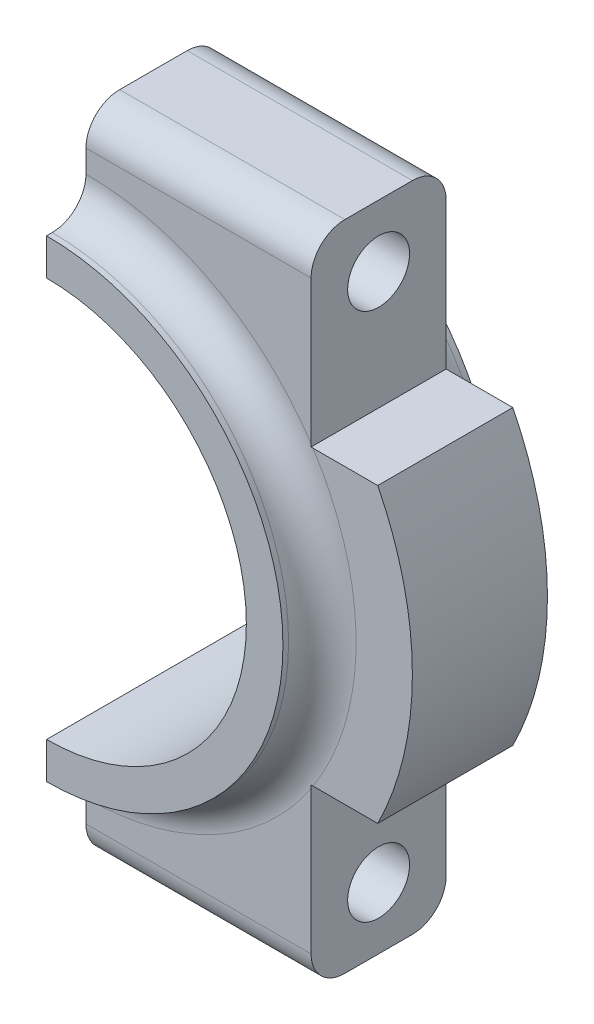
ISO-10303-21;
HEADER;
FILE_DESCRIPTION(('STEP AP214'),'2;1');
FILE_NAME('part.step','',(''),(''),'','','');
FILE_SCHEMA(('AUTOMOTIVE_DESIGN { 1 0 10303 214 1 1 1 1 }'));
ENDSEC;
DATA;
#1=APPLICATION_CONTEXT('core data for automotive mechanical design processes');
#2=APPLICATION_PROTOCOL_DEFINITION('international standard','automotive_design',2000,#1);
#3=PRODUCT_CONTEXT('',#1,'mechanical');
#4=PRODUCT('Part','Part','',(#3));
#5=PRODUCT_RELATED_PRODUCT_CATEGORY('part','',(#4));
#6=PRODUCT_DEFINITION_FORMATION('','',#4);
#7=PRODUCT_DEFINITION_CONTEXT('part definition',#1,'design');
#8=PRODUCT_DEFINITION('design','',#6,#7);
#9=PRODUCT_DEFINITION_SHAPE('','',#8);
#10=(LENGTH_UNIT() NAMED_UNIT(*) SI_UNIT(.MILLI.,.METRE.));
#11=(NAMED_UNIT(*) PLANE_ANGLE_UNIT() SI_UNIT($,.RADIAN.));
#12=(NAMED_UNIT(*) SI_UNIT($,.STERADIAN.) SOLID_ANGLE_UNIT());
#13=UNCERTAINTY_MEASURE_WITH_UNIT(LENGTH_MEASURE(1.E-05),#10,'distance_accuracy_value','');
#14=(GEOMETRIC_REPRESENTATION_CONTEXT(3) GLOBAL_UNCERTAINTY_ASSIGNED_CONTEXT((#13)) GLOBAL_UNIT_ASSIGNED_CONTEXT((#10,
#11,#12)) REPRESENTATION_CONTEXT('',''));
#15=CARTESIAN_POINT('',(0.,0.,0.));
#16=DIRECTION('',(0.,0.,1.));
#17=DIRECTION('',(1.,0.,0.));
#18=AXIS2_PLACEMENT_3D('',#15,#16,#17);
#19=CARTESIAN_POINT('',(0.,0.,-6.));
#20=DIRECTION('',(0.,0.,1.));
#21=DIRECTION('',(1.,0.,0.));
#22=AXIS2_PLACEMENT_3D('',#19,#20,#21);
#23=PLANE('',#22);
#24=DIRECTION('',(0.,1.,0.));
#25=VECTOR('',#24,1.);
#26=CARTESIAN_POINT('',(20.,-29.,-6.));
#27=LINE('',#26,#25);
#28=CARTESIAN_POINT('',(20.,-26.,-6.));
#29=VERTEX_POINT('',#28);
#30=CARTESIAN_POINT('',(20.,-13.2664991614216,-6.));
#31=VERTEX_POINT('',#30);
#32=EDGE_CURVE('E289',#29,#31,#27,.T.);
#33=ORIENTED_EDGE('',*,*,#32,.F.);
#34=DIRECTION('',(1.,0.,0.));
#35=VECTOR('',#34,1.);
#36=CARTESIAN_POINT('',(0.,-26.,-6.));
#37=LINE('',#36,#35);
#38=CARTESIAN_POINT('',(0.,-26.,-6.));
#39=VERTEX_POINT('',#38);
#40=EDGE_CURVE('E467',#29,#39,#37,.F.);
#41=ORIENTED_EDGE('',*,*,#40,.T.);
#42=DIRECTION('',(0.,-1.,0.));
#43=VECTOR('',#42,1.);
#44=CARTESIAN_POINT('',(0.,-17.75,-6.));
#45=LINE('',#44,#43);
#46=CARTESIAN_POINT('',(0.,-24.,-6.));
#47=VERTEX_POINT('',#46);
#48=EDGE_CURVE('E285',#47,#39,#45,.T.);
#49=ORIENTED_EDGE('',*,*,#48,.F.);
#50=CARTESIAN_POINT('',(0.,0.,-6.));
#51=DIRECTION('',(0.,0.,1.));
#52=DIRECTION('',(1.,0.,0.));
#53=AXIS2_PLACEMENT_3D('',#50,#51,#52);
#54=CIRCLE('',#53,24.);
#55=EDGE_CURVE('E470',#47,#31,#54,.T.);
#56=ORIENTED_EDGE('',*,*,#55,.T.);
#57=EDGE_LOOP('',(#33,#41,#49,#56));
#58=FACE_BOUND('',#57,.T.);
#59=ADVANCED_FACE('F39',(#58),#23,.F.);
#60=DIRECTION('',(1.,0.,0.));
#61=VECTOR('',#60,1.);
#62=CARTESIAN_POINT('',(20.,-13.,-6.));
#63=LINE('',#62,#61);
#64=CARTESIAN_POINT('',(20.174241001832,-13.,-6.));
#65=VERTEX_POINT('',#64);
#66=CARTESIAN_POINT('',(25.9229627936314,-13.,-6.));
#67=VERTEX_POINT('',#66);
#68=EDGE_CURVE('E288',#65,#67,#63,.T.);
#69=ORIENTED_EDGE('',*,*,#68,.F.);
#70=CARTESIAN_POINT('',(0.,0.,-6.));
#71=DIRECTION('',(0.,0.,1.));
#72=DIRECTION('',(1.,0.,0.));
#73=AXIS2_PLACEMENT_3D('',#70,#71,#72);
#74=CIRCLE('',#73,24.);
#75=CARTESIAN_POINT('',(20.174241001832,13.,-6.));
#76=VERTEX_POINT('',#75);
#77=EDGE_CURVE('E475',#65,#76,#74,.T.);
#78=ORIENTED_EDGE('',*,*,#77,.T.);
#79=DIRECTION('',(-1.,0.,0.));
#80=VECTOR('',#79,1.);
#81=CARTESIAN_POINT('',(20.,13.,-6.));
#82=LINE('',#81,#80);
#83=CARTESIAN_POINT('',(25.9229627936314,13.,-6.));
#84=VERTEX_POINT('',#83);
#85=EDGE_CURVE('E291',#84,#76,#82,.T.);
#86=ORIENTED_EDGE('',*,*,#85,.F.);
#87=CARTESIAN_POINT('',(0.,0.,-6.));
#88=DIRECTION('',(0.,0.,1.));
#89=DIRECTION('',(1.,0.,0.));
#90=AXIS2_PLACEMENT_3D('',#87,#88,#89);
#91=CIRCLE('',#90,29.);
#92=EDGE_CURVE('E293',#67,#84,#91,.T.);
#93=ORIENTED_EDGE('',*,*,#92,.F.);
#94=EDGE_LOOP('',(#69,#78,#86,#93));
#95=FACE_BOUND('',#94,.T.);
#96=ADVANCED_FACE('F424',(#95),#23,.F.);
#97=CARTESIAN_POINT('',(0.,0.,6.));
#98=DIRECTION('',(0.,0.,1.));
#99=DIRECTION('',(1.,0.,0.));
#100=AXIS2_PLACEMENT_3D('',#97,#98,#99);
#101=PLANE('',#100);
#102=DIRECTION('',(0.,1.,0.));
#103=VECTOR('',#102,1.);
#104=CARTESIAN_POINT('',(20.,29.,6.));
#105=LINE('',#104,#103);
#106=CARTESIAN_POINT('',(20.,13.2664991614216,6.));
#107=VERTEX_POINT('',#106);
#108=CARTESIAN_POINT('',(20.,26.,6.));
#109=VERTEX_POINT('',#108);
#110=EDGE_CURVE('E280',#107,#109,#105,.T.);
#111=ORIENTED_EDGE('',*,*,#110,.T.);
#112=DIRECTION('',(-1.,0.,0.));
#113=VECTOR('',#112,1.);
#114=CARTESIAN_POINT('',(0.,26.,6.));
#115=LINE('',#114,#113);
#116=CARTESIAN_POINT('',(0.,26.,6.));
#117=VERTEX_POINT('',#116);
#118=EDGE_CURVE('E469',#109,#117,#115,.T.);
#119=ORIENTED_EDGE('',*,*,#118,.T.);
#120=DIRECTION('',(0.,-1.,0.));
#121=VECTOR('',#120,1.);
#122=CARTESIAN_POINT('',(0.,29.,6.));
#123=LINE('',#122,#121);
#124=CARTESIAN_POINT('',(0.,24.,6.));
#125=VERTEX_POINT('',#124);
#126=EDGE_CURVE('E261',#117,#125,#123,.T.);
#127=ORIENTED_EDGE('',*,*,#126,.T.);
#128=CARTESIAN_POINT('',(0.,0.,6.));
#129=DIRECTION('',(0.,0.,1.));
#130=DIRECTION('',(1.,0.,0.));
#131=AXIS2_PLACEMENT_3D('',#128,#129,#130);
#132=CIRCLE('',#131,24.);
#133=EDGE_CURVE('E326',#125,#107,#132,.F.);
#134=ORIENTED_EDGE('',*,*,#133,.T.);
#135=EDGE_LOOP('',(#111,#119,#127,#134));
#136=FACE_BOUND('',#135,.T.);
#137=ADVANCED_FACE('F433',(#136),#101,.T.);
#138=DIRECTION('',(-1.,0.,0.));
#139=VECTOR('',#138,1.);
#140=CARTESIAN_POINT('',(20.,13.,6.));
#141=LINE('',#140,#139);
#142=CARTESIAN_POINT('',(25.9229627936314,13.,6.));
#143=VERTEX_POINT('',#142);
#144=CARTESIAN_POINT('',(20.174241001832,13.,6.));
#145=VERTEX_POINT('',#144);
#146=EDGE_CURVE('E274',#143,#145,#141,.T.);
#147=ORIENTED_EDGE('',*,*,#146,.T.);
#148=CARTESIAN_POINT('',(0.,0.,6.));
#149=DIRECTION('',(0.,0.,1.));
#150=DIRECTION('',(1.,0.,0.));
#151=AXIS2_PLACEMENT_3D('',#148,#149,#150);
#152=CIRCLE('',#151,24.);
#153=CARTESIAN_POINT('',(20.174241001832,-13.,6.));
#154=VERTEX_POINT('',#153);
#155=EDGE_CURVE('E323',#145,#154,#152,.F.);
#156=ORIENTED_EDGE('',*,*,#155,.T.);
#157=DIRECTION('',(1.,0.,0.));
#158=VECTOR('',#157,1.);
#159=CARTESIAN_POINT('',(20.,-13.,6.));
#160=LINE('',#159,#158);
#161=CARTESIAN_POINT('',(25.9229627936314,-13.,6.));
#162=VERTEX_POINT('',#161);
#163=EDGE_CURVE('E267',#154,#162,#160,.T.);
#164=ORIENTED_EDGE('',*,*,#163,.T.);
#165=CARTESIAN_POINT('',(0.,0.,6.));
#166=DIRECTION('',(0.,0.,1.));
#167=DIRECTION('',(1.,0.,0.));
#168=AXIS2_PLACEMENT_3D('',#165,#166,#167);
#169=CIRCLE('',#168,29.);
#170=EDGE_CURVE('E275',#162,#143,#169,.T.);
#171=ORIENTED_EDGE('',*,*,#170,.T.);
#172=EDGE_LOOP('',(#147,#156,#164,#171));
#173=FACE_BOUND('',#172,.T.);
#174=ADVANCED_FACE('F448',(#173),#101,.T.);
#175=CARTESIAN_POINT('',(0.,29.,6.));
#176=DIRECTION('',(1.,0.,0.));
#177=DIRECTION('',(0.,0.,-1.));
#178=AXIS2_PLACEMENT_3D('',#175,#176,#177);
#179=PLANE('',#178);
#180=CARTESIAN_POINT('',(0.,23.5,0.));
#181=DIRECTION('',(1.,0.,0.));
#182=DIRECTION('',(0.,1.,0.));
#183=AXIS2_PLACEMENT_3D('',#180,#181,#182);
#184=CIRCLE('',#183,2.75);
#185=CARTESIAN_POINT('',(0.,26.25,0.));
#186=VERTEX_POINT('',#185);
#187=EDGE_CURVE('E249',#186,#186,#184,.T.);
#188=ORIENTED_EDGE('',*,*,#187,.T.);
#189=EDGE_LOOP('',(#188));
#190=FACE_BOUND('',#189,.T.);
#191=ORIENTED_EDGE('',*,*,#126,.F.);
#192=CARTESIAN_POINT('',(0.,26.,3.));
#193=DIRECTION('',(1.,0.,0.));
#194=DIRECTION('',(0.,0.,-1.));
#195=AXIS2_PLACEMENT_3D('',#192,#193,#194);
#196=CIRCLE('',#195,3.);
#197=CARTESIAN_POINT('',(0.,29.,3.));
#198=VERTEX_POINT('',#197);
#199=EDGE_CURVE('E478',#117,#198,#196,.F.);
#200=ORIENTED_EDGE('',*,*,#199,.T.);
#201=DIRECTION('',(0.,0.,-1.));
#202=VECTOR('',#201,1.);
#203=CARTESIAN_POINT('',(0.,29.,6.));
#204=LINE('',#203,#202);
#205=CARTESIAN_POINT('',(0.,29.,-3.));
#206=VERTEX_POINT('',#205);
#207=EDGE_CURVE('E278',#198,#206,#204,.T.);
#208=ORIENTED_EDGE('',*,*,#207,.T.);
#209=CARTESIAN_POINT('',(0.,26.,-3.));
#210=DIRECTION('',(1.,0.,0.));
#211=DIRECTION('',(0.,0.,-1.));
#212=AXIS2_PLACEMENT_3D('',#209,#210,#211);
#213=CIRCLE('',#212,3.);
#214=CARTESIAN_POINT('',(0.,26.,-6.));
#215=VERTEX_POINT('',#214);
#216=EDGE_CURVE('E465',#206,#215,#213,.F.);
#217=ORIENTED_EDGE('',*,*,#216,.T.);
#218=DIRECTION('',(0.,-1.,0.));
#219=VECTOR('',#218,1.);
#220=CARTESIAN_POINT('',(0.,29.,-6.));
#221=LINE('',#220,#219);
#222=CARTESIAN_POINT('',(0.,24.,-6.));
#223=VERTEX_POINT('',#222);
#224=EDGE_CURVE('E254',#215,#223,#221,.T.);
#225=ORIENTED_EDGE('',*,*,#224,.T.);
#226=CARTESIAN_POINT('',(0.,24.,-9.));
#227=DIRECTION('',(1.,0.,0.));
#228=DIRECTION('',(0.,0.,-1.));
#229=AXIS2_PLACEMENT_3D('',#226,#227,#228);
#230=CIRCLE('',#229,3.);
#231=CARTESIAN_POINT('',(0.,21.,-9.));
#232=VERTEX_POINT('',#231);
#233=EDGE_CURVE('E48',#223,#232,#230,.T.);
#234=ORIENTED_EDGE('',*,*,#233,.T.);
#235=DIRECTION('',(0.,0.,1.));
#236=VECTOR('',#235,1.);
#237=CARTESIAN_POINT('',(0.,21.,-9.5));
#238=LINE('',#237,#236);
#239=CARTESIAN_POINT('',(0.,21.,-9.5));
#240=VERTEX_POINT('',#239);
#241=EDGE_CURVE('E215',#240,#232,#238,.T.);
#242=ORIENTED_EDGE('',*,*,#241,.F.);
#243=DIRECTION('',(0.,-1.,0.));
#244=VECTOR('',#243,1.);
#245=CARTESIAN_POINT('',(0.,17.75,-9.5));
#246=LINE('',#245,#244);
#247=CARTESIAN_POINT('',(0.,17.75,-9.5));
#248=VERTEX_POINT('',#247);
#249=EDGE_CURVE('E224',#240,#248,#246,.T.);
#250=ORIENTED_EDGE('',*,*,#249,.T.);
#251=DIRECTION('',(0.,0.,-1.));
#252=VECTOR('',#251,1.);
#253=CARTESIAN_POINT('',(0.,17.75,6.));
#254=LINE('',#253,#252);
#255=CARTESIAN_POINT('',(0.,17.75,9.5));
#256=VERTEX_POINT('',#255);
#257=EDGE_CURVE('E319',#256,#248,#254,.T.);
#258=ORIENTED_EDGE('',*,*,#257,.F.);
#259=DIRECTION('',(0.,-1.,0.));
#260=VECTOR('',#259,1.);
#261=CARTESIAN_POINT('',(0.,17.75,9.5));
#262=LINE('',#261,#260);
#263=CARTESIAN_POINT('',(0.,21.,9.5));
#264=VERTEX_POINT('',#263);
#265=EDGE_CURVE('E232',#264,#256,#262,.T.);
#266=ORIENTED_EDGE('',*,*,#265,.F.);
#267=DIRECTION('',(0.,0.,-1.));
#268=VECTOR('',#267,1.);
#269=CARTESIAN_POINT('',(0.,21.,9.5));
#270=LINE('',#269,#268);
#271=CARTESIAN_POINT('',(0.,21.,9.));
#272=VERTEX_POINT('',#271);
#273=EDGE_CURVE('E246',#264,#272,#270,.T.);
#274=ORIENTED_EDGE('',*,*,#273,.T.);
#275=CARTESIAN_POINT('',(0.,24.,9.));
#276=DIRECTION('',(1.,0.,0.));
#277=DIRECTION('',(0.,0.,-1.));
#278=AXIS2_PLACEMENT_3D('',#275,#276,#277);
#279=CIRCLE('',#278,3.);
#280=EDGE_CURVE('E328',#272,#125,#279,.T.);
#281=ORIENTED_EDGE('',*,*,#280,.T.);
#282=EDGE_LOOP('',(#191,#200,#208,#217,#225,#234,#242,#250,#258,#266,#274,#281));
#283=FACE_BOUND('',#282,.T.);
#284=ADVANCED_FACE('F357',(#190,#283),#179,.F.);
#285=CARTESIAN_POINT('',(0.,0.,6.));
#286=DIRECTION('',(0.,0.,-1.));
#287=DIRECTION('',(-1.,0.,0.));
#288=AXIS2_PLACEMENT_3D('',#285,#286,#287);
#289=CYLINDRICAL_SURFACE('',#288,17.75);
#290=ORIENTED_EDGE('',*,*,#257,.T.);
#291=CARTESIAN_POINT('',(0.,0.,-9.5));
#292=DIRECTION('',(0.,0.,-1.));
#293=DIRECTION('',(1.,0.,0.));
#294=AXIS2_PLACEMENT_3D('',#291,#292,#293);
#295=CIRCLE('',#294,17.75);
#296=CARTESIAN_POINT('',(0.,-17.75,-9.5));
#297=VERTEX_POINT('',#296);
#298=EDGE_CURVE('E227',#248,#297,#295,.T.);
#299=ORIENTED_EDGE('',*,*,#298,.T.);
#300=DIRECTION('',(0.,0.,-1.));
#301=VECTOR('',#300,1.);
#302=CARTESIAN_POINT('',(0.,-17.75,6.));
#303=LINE('',#302,#301);
#304=CARTESIAN_POINT('',(0.,-17.75,9.5));
#305=VERTEX_POINT('',#304);
#306=EDGE_CURVE('E228',#305,#297,#303,.T.);
#307=ORIENTED_EDGE('',*,*,#306,.F.);
#308=CARTESIAN_POINT('',(0.,0.,9.5));
#309=DIRECTION('',(0.,0.,-1.));
#310=DIRECTION('',(1.,0.,0.));
#311=AXIS2_PLACEMENT_3D('',#308,#309,#310);
#312=CIRCLE('',#311,17.75);
#313=EDGE_CURVE('E238',#256,#305,#312,.T.);
#314=ORIENTED_EDGE('',*,*,#313,.F.);
#315=EDGE_LOOP('',(#290,#299,#307,#314));
#316=FACE_BOUND('',#315,.T.);
#317=ADVANCED_FACE('F559',(#316),#289,.F.);
#318=CARTESIAN_POINT('',(0.,-17.75,6.));
#319=DIRECTION('',(1.,0.,0.));
#320=DIRECTION('',(0.,0.,-1.));
#321=AXIS2_PLACEMENT_3D('',#318,#319,#320);
#322=PLANE('',#321);
#323=CARTESIAN_POINT('',(0.,-23.5,0.));
#324=DIRECTION('',(1.,0.,0.));
#325=DIRECTION('',(0.,-1.,0.));
#326=AXIS2_PLACEMENT_3D('',#323,#324,#325);
#327=CIRCLE('',#326,2.75);
#328=CARTESIAN_POINT('',(0.,-26.25,0.));
#329=VERTEX_POINT('',#328);
#330=EDGE_CURVE('E260',#329,#329,#327,.T.);
#331=ORIENTED_EDGE('',*,*,#330,.T.);
#332=EDGE_LOOP('',(#331));
#333=FACE_BOUND('',#332,.T.);
#334=DIRECTION('',(0.,0.,-1.));
#335=VECTOR('',#334,1.);
#336=CARTESIAN_POINT('',(0.,-29.,6.));
#337=LINE('',#336,#335);
#338=CARTESIAN_POINT('',(0.,-29.,3.));
#339=VERTEX_POINT('',#338);
#340=CARTESIAN_POINT('',(0.,-29.,-3.));
#341=VERTEX_POINT('',#340);
#342=EDGE_CURVE('E313',#339,#341,#337,.T.);
#343=ORIENTED_EDGE('',*,*,#342,.F.);
#344=CARTESIAN_POINT('',(0.,-26.,3.));
#345=DIRECTION('',(1.,0.,0.));
#346=DIRECTION('',(0.,0.,-1.));
#347=AXIS2_PLACEMENT_3D('',#344,#345,#346);
#348=CIRCLE('',#347,3.);
#349=CARTESIAN_POINT('',(0.,-26.,6.));
#350=VERTEX_POINT('',#349);
#351=EDGE_CURVE('E528',#339,#350,#348,.F.);
#352=ORIENTED_EDGE('',*,*,#351,.T.);
#353=DIRECTION('',(0.,-1.,0.));
#354=VECTOR('',#353,1.);
#355=CARTESIAN_POINT('',(0.,-17.75,6.));
#356=LINE('',#355,#354);
#357=CARTESIAN_POINT('',(0.,-24.,6.));
#358=VERTEX_POINT('',#357);
#359=EDGE_CURVE('E263',#358,#350,#356,.T.);
#360=ORIENTED_EDGE('',*,*,#359,.F.);
#361=CARTESIAN_POINT('',(0.,-24.,9.));
#362=DIRECTION('',(1.,0.,0.));
#363=DIRECTION('',(0.,0.,-1.));
#364=AXIS2_PLACEMENT_3D('',#361,#362,#363);
#365=CIRCLE('',#364,3.);
#366=CARTESIAN_POINT('',(0.,-21.,9.));
#367=VERTEX_POINT('',#366);
#368=EDGE_CURVE('E512',#358,#367,#365,.T.);
#369=ORIENTED_EDGE('',*,*,#368,.T.);
#370=DIRECTION('',(0.,0.,-1.));
#371=VECTOR('',#370,1.);
#372=CARTESIAN_POINT('',(0.,-21.,9.5));
#373=LINE('',#372,#371);
#374=CARTESIAN_POINT('',(0.,-21.,9.5));
#375=VERTEX_POINT('',#374);
#376=EDGE_CURVE('E243',#375,#367,#373,.T.);
#377=ORIENTED_EDGE('',*,*,#376,.F.);
#378=DIRECTION('',(0.,-1.,0.));
#379=VECTOR('',#378,1.);
#380=CARTESIAN_POINT('',(0.,-17.75,9.5));
#381=LINE('',#380,#379);
#382=EDGE_CURVE('E241',#305,#375,#381,.T.);
#383=ORIENTED_EDGE('',*,*,#382,.F.);
#384=ORIENTED_EDGE('',*,*,#306,.T.);
#385=DIRECTION('',(0.,-1.,0.));
#386=VECTOR('',#385,1.);
#387=CARTESIAN_POINT('',(0.,-17.75,-9.5));
#388=LINE('',#387,#386);
#389=CARTESIAN_POINT('',(0.,-21.,-9.5));
#390=VERTEX_POINT('',#389);
#391=EDGE_CURVE('E220',#297,#390,#388,.T.);
#392=ORIENTED_EDGE('',*,*,#391,.T.);
#393=DIRECTION('',(0.,0.,1.));
#394=VECTOR('',#393,1.);
#395=CARTESIAN_POINT('',(0.,-21.,-9.5));
#396=LINE('',#395,#394);
#397=CARTESIAN_POINT('',(0.,-21.,-9.));
#398=VERTEX_POINT('',#397);
#399=EDGE_CURVE('E197',#390,#398,#396,.T.);
#400=ORIENTED_EDGE('',*,*,#399,.T.);
#401=CARTESIAN_POINT('',(0.,-24.,-9.));
#402=DIRECTION('',(1.,0.,0.));
#403=DIRECTION('',(0.,0.,-1.));
#404=AXIS2_PLACEMENT_3D('',#401,#402,#403);
#405=CIRCLE('',#404,3.);
#406=EDGE_CURVE('E11',#398,#47,#405,.T.);
#407=ORIENTED_EDGE('',*,*,#406,.T.);
#408=ORIENTED_EDGE('',*,*,#48,.T.);
#409=CARTESIAN_POINT('',(0.,-26.,-3.));
#410=DIRECTION('',(1.,0.,0.));
#411=DIRECTION('',(0.,0.,-1.));
#412=AXIS2_PLACEMENT_3D('',#409,#410,#411);
#413=CIRCLE('',#412,3.);
#414=EDGE_CURVE('E526',#39,#341,#413,.F.);
#415=ORIENTED_EDGE('',*,*,#414,.T.);
#416=EDGE_LOOP('',(#343,#352,#360,#369,#377,#383,#384,#392,#400,#407,#408,#415));
#417=FACE_BOUND('',#416,.T.);
#418=ADVANCED_FACE('F223',(#333,#417),#322,.F.);
#419=CARTESIAN_POINT('',(0.,-29.,6.));
#420=DIRECTION('',(0.,1.,0.));
#421=DIRECTION('',(0.,0.,1.));
#422=AXIS2_PLACEMENT_3D('',#419,#420,#421);
#423=PLANE('',#422);
#424=DIRECTION('',(0.,0.,-1.));
#425=VECTOR('',#424,1.);
#426=CARTESIAN_POINT('',(20.,-29.,6.));
#427=LINE('',#426,#425);
#428=CARTESIAN_POINT('',(20.,-29.,3.));
#429=VERTEX_POINT('',#428);
#430=CARTESIAN_POINT('',(20.,-29.,-3.));
#431=VERTEX_POINT('',#430);
#432=EDGE_CURVE('E311',#429,#431,#427,.T.);
#433=ORIENTED_EDGE('',*,*,#432,.F.);
#434=DIRECTION('',(1.,0.,0.));
#435=VECTOR('',#434,1.);
#436=CARTESIAN_POINT('',(0.,-29.,3.));
#437=LINE('',#436,#435);
#438=EDGE_CURVE('E522',#429,#339,#437,.F.);
#439=ORIENTED_EDGE('',*,*,#438,.T.);
#440=ORIENTED_EDGE('',*,*,#342,.T.);
#441=DIRECTION('',(1.,0.,0.));
#442=VECTOR('',#441,1.);
#443=CARTESIAN_POINT('',(0.,-29.,-3.));
#444=LINE('',#443,#442);
#445=EDGE_CURVE('E521',#341,#431,#444,.T.);
#446=ORIENTED_EDGE('',*,*,#445,.T.);
#447=EDGE_LOOP('',(#433,#439,#440,#446));
#448=FACE_BOUND('',#447,.T.);
#449=ADVANCED_FACE('F540',(#448),#423,.F.);
#450=CARTESIAN_POINT('',(20.,-29.,6.));
#451=DIRECTION('',(-1.,0.,0.));
#452=DIRECTION('',(0.,-1.,0.));
#453=AXIS2_PLACEMENT_3D('',#450,#451,#452);
#454=PLANE('',#453);
#455=CARTESIAN_POINT('',(20.,-23.5,0.));
#456=DIRECTION('',(1.,0.,0.));
#457=DIRECTION('',(0.,-1.,0.));
#458=AXIS2_PLACEMENT_3D('',#455,#456,#457);
#459=CIRCLE('',#458,2.75);
#460=CARTESIAN_POINT('',(20.,-26.25,0.));
#461=VERTEX_POINT('',#460);
#462=EDGE_CURVE('E248',#461,#461,#459,.T.);
#463=ORIENTED_EDGE('',*,*,#462,.F.);
#464=EDGE_LOOP('',(#463));
#465=FACE_BOUND('',#464,.T.);
#466=DIRECTION('',(0.,1.,0.));
#467=VECTOR('',#466,1.);
#468=CARTESIAN_POINT('',(20.,-29.,6.));
#469=LINE('',#468,#467);
#470=CARTESIAN_POINT('',(20.,-26.,6.));
#471=VERTEX_POINT('',#470);
#472=CARTESIAN_POINT('',(20.,-13.2664991614216,6.));
#473=VERTEX_POINT('',#472);
#474=EDGE_CURVE('E270',#471,#473,#469,.T.);
#475=ORIENTED_EDGE('',*,*,#474,.F.);
#476=CARTESIAN_POINT('',(20.,-26.,3.));
#477=DIRECTION('',(-1.,0.,0.));
#478=DIRECTION('',(0.,-1.,0.));
#479=AXIS2_PLACEMENT_3D('',#476,#477,#478);
#480=CIRCLE('',#479,3.);
#481=EDGE_CURVE('E518',#471,#429,#480,.F.);
#482=ORIENTED_EDGE('',*,*,#481,.T.);
#483=ORIENTED_EDGE('',*,*,#432,.T.);
#484=CARTESIAN_POINT('',(20.,-26.,-3.));
#485=DIRECTION('',(-1.,0.,0.));
#486=DIRECTION('',(0.,-1.,0.));
#487=AXIS2_PLACEMENT_3D('',#484,#485,#486);
#488=CIRCLE('',#487,3.);
#489=EDGE_CURVE('E517',#431,#29,#488,.F.);
#490=ORIENTED_EDGE('',*,*,#489,.T.);
#491=ORIENTED_EDGE('',*,*,#32,.T.);
#492=CARTESIAN_POINT('',(20.,-13.2664991614216,-6.));
#493=CARTESIAN_POINT('',(20.,-13.2220747115021,-6.0000040632633));
#494=CARTESIAN_POINT('',(20.,-13.1776542160634,-6.00030346054399));
#495=CARTESIAN_POINT('',(20.,-13.0888211622612,-6.00149292276371));
#496=CARTESIAN_POINT('',(20.,-13.0444086038927,-6.00238298732887));
#497=CARTESIAN_POINT('',(20.,-13.,-6.00356838553755));
#498=B_SPLINE_CURVE_WITH_KNOTS('',3,(#492,#493,#494,#495,#496,#497),.UNSPECIFIED.,.F.,.F.,(4,2,
4),(0.,0.133264513220164,0.266528942089409),.UNSPECIFIED.);
#499=CARTESIAN_POINT('',(20.,-13.,-6.00356838553755));
#500=VERTEX_POINT('',#499);
#501=EDGE_CURVE('E399',#31,#500,#498,.T.);
#502=ORIENTED_EDGE('',*,*,#501,.T.);
#503=DIRECTION('',(0.,0.,-1.));
#504=VECTOR('',#503,1.);
#505=CARTESIAN_POINT('',(20.,-13.,6.));
#506=LINE('',#505,#504);
#507=CARTESIAN_POINT('',(20.,-13.,6.00356838553755));
#508=VERTEX_POINT('',#507);
#509=EDGE_CURVE('E64',#508,#500,#506,.T.);
#510=ORIENTED_EDGE('',*,*,#509,.F.);
#511=CARTESIAN_POINT('',(20.,-13.,6.00356838553755));
#512=CARTESIAN_POINT('',(20.,-13.0444086038927,6.00238298732886));
#513=CARTESIAN_POINT('',(20.,-13.0888211622612,6.0014929227637));
#514=CARTESIAN_POINT('',(20.,-13.1776542160633,6.00030346054399));
#515=CARTESIAN_POINT('',(20.,-13.2220747115021,6.0000040632633));
#516=CARTESIAN_POINT('',(20.,-13.2664991614216,6.));
#517=B_SPLINE_CURVE_WITH_KNOTS('',3,(#511,#512,#513,#514,#515,#516),.UNSPECIFIED.,.F.,.F.,(4,2,
4),(0.,0.133264428869243,0.266528942089407),.UNSPECIFIED.);
#518=EDGE_CURVE('E371',#508,#473,#517,.T.);
#519=ORIENTED_EDGE('',*,*,#518,.T.);
#520=EDGE_LOOP('',(#475,#482,#483,#490,#491,#502,#510,#519));
#521=FACE_BOUND('',#520,.T.);
#522=ADVANCED_FACE('F384',(#465,#521),#454,.F.);
#523=CARTESIAN_POINT('',(20.,-13.,6.));
#524=DIRECTION('',(0.,1.,0.));
#525=DIRECTION('',(0.,0.,1.));
#526=AXIS2_PLACEMENT_3D('',#523,#524,#525);
#527=PLANE('',#526);
#528=ORIENTED_EDGE('',*,*,#509,.T.);
#529=CARTESIAN_POINT('',(20.,-13.,-6.00356838553755));
#530=CARTESIAN_POINT('',(20.0290279984839,-13.,-6.00237966920018));
#531=CARTESIAN_POINT('',(20.0580620792593,-13.,-6.00148794557008));
#532=CARTESIAN_POINT('',(20.1161424132001,-13.,-6.00029848356455));
#533=CARTESIAN_POINT('',(20.1451886663687,-13.,-6.00000074534879));
#534=CARTESIAN_POINT('',(20.174241001832,-13.,-6.));
#535=B_SPLINE_CURVE_WITH_KNOTS('',3,(#529,#530,#531,#532,#533,#534),.UNSPECIFIED.,.F.,.F.,(4,2,
4),(0.,0.0871433139003512,0.17428665122816),.UNSPECIFIED.);
#536=EDGE_CURVE('E389',#500,#65,#535,.T.);
#537=ORIENTED_EDGE('',*,*,#536,.T.);
#538=ORIENTED_EDGE('',*,*,#68,.T.);
#539=DIRECTION('',(0.,0.,-1.));
#540=VECTOR('',#539,1.);
#541=CARTESIAN_POINT('',(25.9229627936314,-13.,6.));
#542=LINE('',#541,#540);
#543=EDGE_CURVE('E310',#162,#67,#542,.T.);
#544=ORIENTED_EDGE('',*,*,#543,.F.);
#545=ORIENTED_EDGE('',*,*,#163,.F.);
#546=CARTESIAN_POINT('',(20.174241001832,-13.,6.));
#547=CARTESIAN_POINT('',(20.1451886663687,-13.,6.00000074534879));
#548=CARTESIAN_POINT('',(20.1161424132001,-13.,6.00029848356455));
#549=CARTESIAN_POINT('',(20.0580620792593,-13.,6.00148794557008));
#550=CARTESIAN_POINT('',(20.0290279984839,-13.,6.00237966920018));
#551=CARTESIAN_POINT('',(20.,-13.,6.00356838553755));
#552=B_SPLINE_CURVE_WITH_KNOTS('',3,(#546,#547,#548,#549,#550,#551),.UNSPECIFIED.,.F.,.F.,(4,2,
4),(0.,0.0871433373278087,0.17428665122816),.UNSPECIFIED.);
#553=EDGE_CURVE('E362',#154,#508,#552,.T.);
#554=ORIENTED_EDGE('',*,*,#553,.T.);
#555=EDGE_LOOP('',(#528,#537,#538,#544,#545,#554));
#556=FACE_BOUND('',#555,.T.);
#557=ADVANCED_FACE('F377',(#556),#527,.F.);
#558=CARTESIAN_POINT('',(0.,0.,6.));
#559=DIRECTION('',(0.,0.,-1.));
#560=DIRECTION('',(-1.,0.,0.));
#561=AXIS2_PLACEMENT_3D('',#558,#559,#560);
#562=CYLINDRICAL_SURFACE('',#561,29.);
#563=ORIENTED_EDGE('',*,*,#92,.T.);
#564=DIRECTION('',(0.,0.,-1.));
#565=VECTOR('',#564,1.);
#566=CARTESIAN_POINT('',(25.9229627936314,13.,6.));
#567=LINE('',#566,#565);
#568=EDGE_CURVE('E302',#143,#84,#567,.T.);
#569=ORIENTED_EDGE('',*,*,#568,.F.);
#570=ORIENTED_EDGE('',*,*,#170,.F.);
#571=ORIENTED_EDGE('',*,*,#543,.T.);
#572=EDGE_LOOP('',(#563,#569,#570,#571));
#573=FACE_BOUND('',#572,.T.);
#574=ADVANCED_FACE('F385',(#573),#562,.T.);
#575=CARTESIAN_POINT('',(20.,13.,6.));
#576=DIRECTION('',(0.,-1.,0.));
#577=DIRECTION('',(0.,0.,-1.));
#578=AXIS2_PLACEMENT_3D('',#575,#576,#577);
#579=PLANE('',#578);
#580=ORIENTED_EDGE('',*,*,#85,.T.);
#581=CARTESIAN_POINT('',(20.174241001832,13.,-6.));
#582=CARTESIAN_POINT('',(20.1451886663687,13.,-6.00000074534879));
#583=CARTESIAN_POINT('',(20.1161424132001,13.,-6.00029848356455));
#584=CARTESIAN_POINT('',(20.0580620792593,13.,-6.00148794557008));
#585=CARTESIAN_POINT('',(20.029027998484,13.,-6.00237966920018));
#586=CARTESIAN_POINT('',(20.,13.,-6.00356838553755));
#587=B_SPLINE_CURVE_WITH_KNOTS('',3,(#581,#582,#583,#584,#585,#586),.UNSPECIFIED.,.F.,.F.,(4,2,
4),(0.,0.0871433373278017,0.174286651228146),.UNSPECIFIED.);
#588=CARTESIAN_POINT('',(20.,13.,-6.00356838553755));
#589=VERTEX_POINT('',#588);
#590=EDGE_CURVE('E392',#76,#589,#587,.T.);
#591=ORIENTED_EDGE('',*,*,#590,.T.);
#592=DIRECTION('',(0.,0.,-1.));
#593=VECTOR('',#592,1.);
#594=CARTESIAN_POINT('',(20.,13.,6.));
#595=LINE('',#594,#593);
#596=CARTESIAN_POINT('',(20.,13.,6.00356838553755));
#597=VERTEX_POINT('',#596);
#598=EDGE_CURVE('E54',#597,#589,#595,.T.);
#599=ORIENTED_EDGE('',*,*,#598,.F.);
#600=CARTESIAN_POINT('',(20.,13.,6.00356838553755));
#601=CARTESIAN_POINT('',(20.029027998484,13.,6.00237966920018));
#602=CARTESIAN_POINT('',(20.0580620792593,13.,6.00148794557008));
#603=CARTESIAN_POINT('',(20.1161424132001,13.,6.00029848356455));
#604=CARTESIAN_POINT('',(20.1451886663687,13.,6.0000007453488));
#605=CARTESIAN_POINT('',(20.174241001832,13.,6.));
#606=B_SPLINE_CURVE_WITH_KNOTS('',3,(#600,#601,#602,#603,#604,#605),.UNSPECIFIED.,.F.,.F.,(4,2,
4),(0.,0.0871433139003443,0.174286651228146),.UNSPECIFIED.);
#607=EDGE_CURVE('E338',#597,#145,#606,.T.);
#608=ORIENTED_EDGE('',*,*,#607,.T.);
#609=ORIENTED_EDGE('',*,*,#146,.F.);
#610=ORIENTED_EDGE('',*,*,#568,.T.);
#611=EDGE_LOOP('',(#580,#591,#599,#608,#609,#610));
#612=FACE_BOUND('',#611,.T.);
#613=ADVANCED_FACE('F411',(#612),#579,.F.);
#614=CARTESIAN_POINT('',(20.,29.,6.));
#615=DIRECTION('',(-1.,0.,0.));
#616=DIRECTION('',(0.,-1.,0.));
#617=AXIS2_PLACEMENT_3D('',#614,#615,#616);
#618=PLANE('',#617);
#619=CARTESIAN_POINT('',(20.,23.5,0.));
#620=DIRECTION('',(1.,0.,0.));
#621=DIRECTION('',(0.,1.,0.));
#622=AXIS2_PLACEMENT_3D('',#619,#620,#621);
#623=CIRCLE('',#622,2.75);
#624=CARTESIAN_POINT('',(20.,26.25,0.));
#625=VERTEX_POINT('',#624);
#626=EDGE_CURVE('E251',#625,#625,#623,.T.);
#627=ORIENTED_EDGE('',*,*,#626,.F.);
#628=EDGE_LOOP('',(#627));
#629=FACE_BOUND('',#628,.T.);
#630=DIRECTION('',(0.,0.,-1.));
#631=VECTOR('',#630,1.);
#632=CARTESIAN_POINT('',(20.,29.,6.));
#633=LINE('',#632,#631);
#634=CARTESIAN_POINT('',(20.,29.,3.));
#635=VERTEX_POINT('',#634);
#636=CARTESIAN_POINT('',(20.,29.,-3.));
#637=VERTEX_POINT('',#636);
#638=EDGE_CURVE('E297',#635,#637,#633,.T.);
#639=ORIENTED_EDGE('',*,*,#638,.F.);
#640=CARTESIAN_POINT('',(20.,26.,3.));
#641=DIRECTION('',(-1.,0.,0.));
#642=DIRECTION('',(0.,-1.,0.));
#643=AXIS2_PLACEMENT_3D('',#640,#641,#642);
#644=CIRCLE('',#643,3.);
#645=EDGE_CURVE('E488',#635,#109,#644,.F.);
#646=ORIENTED_EDGE('',*,*,#645,.T.);
#647=ORIENTED_EDGE('',*,*,#110,.F.);
#648=CARTESIAN_POINT('',(20.,13.2664991614216,6.));
#649=CARTESIAN_POINT('',(20.,13.2220747115021,6.0000040632633));
#650=CARTESIAN_POINT('',(20.,13.1776542160633,6.00030346054399));
#651=CARTESIAN_POINT('',(20.,13.0888211622611,6.00149292276371));
#652=CARTESIAN_POINT('',(20.,13.0444086038927,6.00238298732887));
#653=CARTESIAN_POINT('',(20.,13.,6.00356838553755));
#654=B_SPLINE_CURVE_WITH_KNOTS('',3,(#648,#649,#650,#651,#652,#653),.UNSPECIFIED.,.F.,.F.,(4,2,
4),(0.,0.133264513220156,0.26652894208939),.UNSPECIFIED.);
#655=EDGE_CURVE('E331',#107,#597,#654,.T.);
#656=ORIENTED_EDGE('',*,*,#655,.T.);
#657=ORIENTED_EDGE('',*,*,#598,.T.);
#658=CARTESIAN_POINT('',(20.,13.,-6.00356838553755));
#659=CARTESIAN_POINT('',(20.,13.0444086038927,-6.00238298732886));
#660=CARTESIAN_POINT('',(20.,13.0888211622611,-6.0014929227637));
#661=CARTESIAN_POINT('',(20.,13.1776542160633,-6.00030346054399));
#662=CARTESIAN_POINT('',(20.,13.2220747115021,-6.0000040632633));
#663=CARTESIAN_POINT('',(20.,13.2664991614216,-6.));
#664=B_SPLINE_CURVE_WITH_KNOTS('',3,(#658,#659,#660,#661,#662,#663),.UNSPECIFIED.,.F.,.F.,(4,2,
4),(0.,0.133264428869234,0.266528942089388),.UNSPECIFIED.);
#665=CARTESIAN_POINT('',(20.,13.2664991614216,-6.));
#666=VERTEX_POINT('',#665);
#667=EDGE_CURVE('E410',#589,#666,#664,.T.);
#668=ORIENTED_EDGE('',*,*,#667,.T.);
#669=DIRECTION('',(0.,1.,0.));
#670=VECTOR('',#669,1.);
#671=CARTESIAN_POINT('',(20.,29.,-6.));
#672=LINE('',#671,#670);
#673=CARTESIAN_POINT('',(20.,26.,-6.));
#674=VERTEX_POINT('',#673);
#675=EDGE_CURVE('E262',#666,#674,#672,.T.);
#676=ORIENTED_EDGE('',*,*,#675,.T.);
#677=CARTESIAN_POINT('',(20.,26.,-3.));
#678=DIRECTION('',(-1.,0.,0.));
#679=DIRECTION('',(0.,-1.,0.));
#680=AXIS2_PLACEMENT_3D('',#677,#678,#679);
#681=CIRCLE('',#680,3.);
#682=EDGE_CURVE('E462',#674,#637,#681,.F.);
#683=ORIENTED_EDGE('',*,*,#682,.T.);
#684=EDGE_LOOP('',(#639,#646,#647,#656,#657,#668,#676,#683));
#685=FACE_BOUND('',#684,.T.);
#686=ADVANCED_FACE('F346',(#629,#685),#618,.F.);
#687=CARTESIAN_POINT('',(0.,29.,6.));
#688=DIRECTION('',(0.,-1.,0.));
#689=DIRECTION('',(0.,0.,-1.));
#690=AXIS2_PLACEMENT_3D('',#687,#688,#689);
#691=PLANE('',#690);
#692=ORIENTED_EDGE('',*,*,#207,.F.);
#693=DIRECTION('',(-1.,0.,0.));
#694=VECTOR('',#693,1.);
#695=CARTESIAN_POINT('',(20.,29.,3.));
#696=LINE('',#695,#694);
#697=EDGE_CURVE('E485',#198,#635,#696,.F.);
#698=ORIENTED_EDGE('',*,*,#697,.T.);
#699=ORIENTED_EDGE('',*,*,#638,.T.);
#700=DIRECTION('',(-1.,0.,0.));
#701=VECTOR('',#700,1.);
#702=CARTESIAN_POINT('',(0.,29.,-3.));
#703=LINE('',#702,#701);
#704=EDGE_CURVE('E484',#637,#206,#703,.T.);
#705=ORIENTED_EDGE('',*,*,#704,.T.);
#706=EDGE_LOOP('',(#692,#698,#699,#705));
#707=FACE_BOUND('',#706,.T.);
#708=ADVANCED_FACE('F417',(#707),#691,.F.);
#709=ORIENTED_EDGE('',*,*,#359,.T.);
#710=DIRECTION('',(1.,0.,0.));
#711=VECTOR('',#710,1.);
#712=CARTESIAN_POINT('',(20.,-26.,6.));
#713=LINE('',#712,#711);
#714=EDGE_CURVE('E515',#350,#471,#713,.T.);
#715=ORIENTED_EDGE('',*,*,#714,.T.);
#716=ORIENTED_EDGE('',*,*,#474,.T.);
#717=CARTESIAN_POINT('',(0.,0.,6.));
#718=DIRECTION('',(0.,0.,1.));
#719=DIRECTION('',(1.,0.,0.));
#720=AXIS2_PLACEMENT_3D('',#717,#718,#719);
#721=CIRCLE('',#720,24.);
#722=EDGE_CURVE('E324',#473,#358,#721,.F.);
#723=ORIENTED_EDGE('',*,*,#722,.T.);
#724=EDGE_LOOP('',(#709,#715,#716,#723));
#725=FACE_BOUND('',#724,.T.);
#726=ADVANCED_FACE('F437',(#725),#101,.T.);
#727=ORIENTED_EDGE('',*,*,#224,.F.);
#728=DIRECTION('',(-1.,0.,0.));
#729=VECTOR('',#728,1.);
#730=CARTESIAN_POINT('',(0.,26.,-6.));
#731=LINE('',#730,#729);
#732=EDGE_CURVE('E451',#215,#674,#731,.F.);
#733=ORIENTED_EDGE('',*,*,#732,.T.);
#734=ORIENTED_EDGE('',*,*,#675,.F.);
#735=CARTESIAN_POINT('',(0.,0.,-6.));
#736=DIRECTION('',(0.,0.,1.));
#737=DIRECTION('',(1.,0.,0.));
#738=AXIS2_PLACEMENT_3D('',#735,#736,#737);
#739=CIRCLE('',#738,24.);
#740=EDGE_CURVE('E459',#666,#223,#739,.T.);
#741=ORIENTED_EDGE('',*,*,#740,.T.);
#742=EDGE_LOOP('',(#727,#733,#734,#741));
#743=FACE_BOUND('',#742,.T.);
#744=ADVANCED_FACE('F426',(#743),#23,.F.);
#745=CARTESIAN_POINT('',(0.,23.5,0.));
#746=DIRECTION('',(1.,0.,0.));
#747=DIRECTION('',(0.,1.,0.));
#748=AXIS2_PLACEMENT_3D('',#745,#746,#747);
#749=CYLINDRICAL_SURFACE('',#748,2.75);
#750=ORIENTED_EDGE('',*,*,#187,.F.);
#751=EDGE_LOOP('',(#750));
#752=FACE_BOUND('',#751,.T.);
#753=ORIENTED_EDGE('',*,*,#626,.T.);
#754=EDGE_LOOP('',(#753));
#755=FACE_BOUND('',#754,.T.);
#756=ADVANCED_FACE('F438',(#752,#755),#749,.F.);
#757=CARTESIAN_POINT('',(0.,-23.5,0.));
#758=DIRECTION('',(1.,0.,0.));
#759=DIRECTION('',(0.,1.,0.));
#760=AXIS2_PLACEMENT_3D('',#757,#758,#759);
#761=CYLINDRICAL_SURFACE('',#760,2.75);
#762=ORIENTED_EDGE('',*,*,#330,.F.);
#763=EDGE_LOOP('',(#762));
#764=FACE_BOUND('',#763,.T.);
#765=ORIENTED_EDGE('',*,*,#462,.T.);
#766=EDGE_LOOP('',(#765));
#767=FACE_BOUND('',#766,.T.);
#768=ADVANCED_FACE('F447',(#764,#767),#761,.F.);
#769=CARTESIAN_POINT('',(0.,0.,9.5));
#770=DIRECTION('',(0.,0.,-1.));
#771=DIRECTION('',(-1.,0.,0.));
#772=AXIS2_PLACEMENT_3D('',#769,#770,#771);
#773=CYLINDRICAL_SURFACE('',#772,21.);
#774=ORIENTED_EDGE('',*,*,#376,.T.);
#775=CARTESIAN_POINT('',(0.,0.,9.));
#776=DIRECTION('',(0.,0.,1.));
#777=DIRECTION('',(1.,0.,0.));
#778=AXIS2_PLACEMENT_3D('',#775,#776,#777);
#779=CIRCLE('',#778,21.);
#780=EDGE_CURVE('E318',#367,#272,#779,.T.);
#781=ORIENTED_EDGE('',*,*,#780,.T.);
#782=ORIENTED_EDGE('',*,*,#273,.F.);
#783=CARTESIAN_POINT('',(0.,0.,9.5));
#784=DIRECTION('',(0.,0.,1.));
#785=DIRECTION('',(1.,0.,0.));
#786=AXIS2_PLACEMENT_3D('',#783,#784,#785);
#787=CIRCLE('',#786,21.);
#788=EDGE_CURVE('E212',#375,#264,#787,.T.);
#789=ORIENTED_EDGE('',*,*,#788,.F.);
#790=EDGE_LOOP('',(#774,#781,#782,#789));
#791=FACE_BOUND('',#790,.T.);
#792=ADVANCED_FACE('F554',(#791),#773,.T.);
#793=CARTESIAN_POINT('',(0.,0.,9.5));
#794=DIRECTION('',(0.,0.,1.));
#795=DIRECTION('',(1.,0.,0.));
#796=AXIS2_PLACEMENT_3D('',#793,#794,#795);
#797=PLANE('',#796);
#798=ORIENTED_EDGE('',*,*,#788,.T.);
#799=ORIENTED_EDGE('',*,*,#265,.T.);
#800=ORIENTED_EDGE('',*,*,#313,.T.);
#801=ORIENTED_EDGE('',*,*,#382,.T.);
#802=EDGE_LOOP('',(#798,#799,#800,#801));
#803=FACE_BOUND('',#802,.T.);
#804=ADVANCED_FACE('F352',(#803),#797,.T.);
#805=CARTESIAN_POINT('',(0.,0.,9.));
#806=DIRECTION('',(0.,0.,1.));
#807=DIRECTION('',(1.,0.,0.));
#808=AXIS2_PLACEMENT_3D('',#805,#806,#807);
#809=TOROIDAL_SURFACE('',#808,24.,3.);
#810=ORIENTED_EDGE('',*,*,#655,.F.);
#811=ORIENTED_EDGE('',*,*,#133,.F.);
#812=ORIENTED_EDGE('',*,*,#280,.F.);
#813=ORIENTED_EDGE('',*,*,#780,.F.);
#814=ORIENTED_EDGE('',*,*,#368,.F.);
#815=ORIENTED_EDGE('',*,*,#722,.F.);
#816=ORIENTED_EDGE('',*,*,#518,.F.);
#817=ORIENTED_EDGE('',*,*,#553,.F.);
#818=ORIENTED_EDGE('',*,*,#155,.F.);
#819=ORIENTED_EDGE('',*,*,#607,.F.);
#820=EDGE_LOOP('',(#810,#811,#812,#813,#814,#815,#816,#817,#818,#819));
#821=FACE_BOUND('',#820,.T.);
#822=ADVANCED_FACE('F347',(#821),#809,.F.);
#823=CARTESIAN_POINT('',(0.,0.,-9.5));
#824=DIRECTION('',(0.,0.,1.));
#825=DIRECTION('',(1.,0.,0.));
#826=AXIS2_PLACEMENT_3D('',#823,#824,#825);
#827=CYLINDRICAL_SURFACE('',#826,21.);
#828=ORIENTED_EDGE('',*,*,#241,.T.);
#829=CARTESIAN_POINT('',(0.,0.,-9.));
#830=DIRECTION('',(0.,0.,1.));
#831=DIRECTION('',(1.,0.,0.));
#832=AXIS2_PLACEMENT_3D('',#829,#830,#831);
#833=CIRCLE('',#832,21.);
#834=EDGE_CURVE('E210',#232,#398,#833,.F.);
#835=ORIENTED_EDGE('',*,*,#834,.T.);
#836=ORIENTED_EDGE('',*,*,#399,.F.);
#837=CARTESIAN_POINT('',(0.,0.,-9.5));
#838=DIRECTION('',(0.,0.,1.));
#839=DIRECTION('',(1.,0.,0.));
#840=AXIS2_PLACEMENT_3D('',#837,#838,#839);
#841=CIRCLE('',#840,21.);
#842=EDGE_CURVE('E203',#390,#240,#841,.T.);
#843=ORIENTED_EDGE('',*,*,#842,.T.);
#844=EDGE_LOOP('',(#828,#835,#836,#843));
#845=FACE_BOUND('',#844,.T.);
#846=ADVANCED_FACE('F205',(#845),#827,.T.);
#847=CARTESIAN_POINT('',(0.,0.,-9.5));
#848=DIRECTION('',(0.,0.,-1.));
#849=DIRECTION('',(1.,0.,0.));
#850=AXIS2_PLACEMENT_3D('',#847,#848,#849);
#851=PLANE('',#850);
#852=ORIENTED_EDGE('',*,*,#842,.F.);
#853=ORIENTED_EDGE('',*,*,#391,.F.);
#854=ORIENTED_EDGE('',*,*,#298,.F.);
#855=ORIENTED_EDGE('',*,*,#249,.F.);
#856=EDGE_LOOP('',(#852,#853,#854,#855));
#857=FACE_BOUND('',#856,.T.);
#858=ADVANCED_FACE('F219',(#857),#851,.T.);
#859=CARTESIAN_POINT('',(0.,-26.,3.));
#860=DIRECTION('',(-1.,0.,0.));
#861=DIRECTION('',(0.,0.,1.));
#862=AXIS2_PLACEMENT_3D('',#859,#860,#861);
#863=CYLINDRICAL_SURFACE('',#862,3.);
#864=ORIENTED_EDGE('',*,*,#351,.F.);
#865=ORIENTED_EDGE('',*,*,#438,.F.);
#866=ORIENTED_EDGE('',*,*,#481,.F.);
#867=ORIENTED_EDGE('',*,*,#714,.F.);
#868=EDGE_LOOP('',(#864,#865,#866,#867));
#869=FACE_BOUND('',#868,.T.);
#870=ADVANCED_FACE('F360',(#869),#863,.T.);
#871=CARTESIAN_POINT('',(0.,-26.,-3.));
#872=DIRECTION('',(1.,0.,0.));
#873=DIRECTION('',(0.,0.,-1.));
#874=AXIS2_PLACEMENT_3D('',#871,#872,#873);
#875=CYLINDRICAL_SURFACE('',#874,3.);
#876=ORIENTED_EDGE('',*,*,#414,.F.);
#877=ORIENTED_EDGE('',*,*,#40,.F.);
#878=ORIENTED_EDGE('',*,*,#489,.F.);
#879=ORIENTED_EDGE('',*,*,#445,.F.);
#880=EDGE_LOOP('',(#876,#877,#878,#879));
#881=FACE_BOUND('',#880,.T.);
#882=ADVANCED_FACE('F544',(#881),#875,.T.);
#883=CARTESIAN_POINT('',(0.,26.,3.));
#884=DIRECTION('',(1.,0.,0.));
#885=DIRECTION('',(0.,0.,-1.));
#886=AXIS2_PLACEMENT_3D('',#883,#884,#885);
#887=CYLINDRICAL_SURFACE('',#886,3.);
#888=ORIENTED_EDGE('',*,*,#645,.F.);
#889=ORIENTED_EDGE('',*,*,#697,.F.);
#890=ORIENTED_EDGE('',*,*,#199,.F.);
#891=ORIENTED_EDGE('',*,*,#118,.F.);
#892=EDGE_LOOP('',(#888,#889,#890,#891));
#893=FACE_BOUND('',#892,.T.);
#894=ADVANCED_FACE('F592',(#893),#887,.T.);
#895=CARTESIAN_POINT('',(0.,26.,-3.));
#896=DIRECTION('',(-1.,0.,0.));
#897=DIRECTION('',(0.,0.,1.));
#898=AXIS2_PLACEMENT_3D('',#895,#896,#897);
#899=CYLINDRICAL_SURFACE('',#898,3.);
#900=ORIENTED_EDGE('',*,*,#682,.F.);
#901=ORIENTED_EDGE('',*,*,#732,.F.);
#902=ORIENTED_EDGE('',*,*,#216,.F.);
#903=ORIENTED_EDGE('',*,*,#704,.F.);
#904=EDGE_LOOP('',(#900,#901,#902,#903));
#905=FACE_BOUND('',#904,.T.);
#906=ADVANCED_FACE('F464',(#905),#899,.T.);
#907=CARTESIAN_POINT('',(0.,0.,-9.));
#908=DIRECTION('',(0.,0.,1.));
#909=DIRECTION('',(1.,0.,0.));
#910=AXIS2_PLACEMENT_3D('',#907,#908,#909);
#911=TOROIDAL_SURFACE('',#910,24.,3.);
#912=ORIENTED_EDGE('',*,*,#406,.F.);
#913=ORIENTED_EDGE('',*,*,#834,.F.);
#914=ORIENTED_EDGE('',*,*,#233,.F.);
#915=ORIENTED_EDGE('',*,*,#740,.F.);
#916=ORIENTED_EDGE('',*,*,#667,.F.);
#917=ORIENTED_EDGE('',*,*,#590,.F.);
#918=ORIENTED_EDGE('',*,*,#77,.F.);
#919=ORIENTED_EDGE('',*,*,#536,.F.);
#920=ORIENTED_EDGE('',*,*,#501,.F.);
#921=ORIENTED_EDGE('',*,*,#55,.F.);
#922=EDGE_LOOP('',(#912,#913,#914,#915,#916,#917,#918,#919,#920,#921));
#923=FACE_BOUND('',#922,.T.);
#924=ADVANCED_FACE('F41',(#923),#911,.F.);
#925=CLOSED_SHELL('',(#59,#96,#137,#174,#284,#317,#418,#449,#522,#557,#574,#613,#686,#708,#726,
#744,#756,#768,#792,#804,#822,#846,#858,#870,#882,#894,#906,#924));
#926=MANIFOLD_SOLID_BREP('B2',#925);
#927=ADVANCED_BREP_SHAPE_REPRESENTATION('',(#18,#926),#14);
#928=SHAPE_DEFINITION_REPRESENTATION(#9,#927);
ENDSEC;
END-ISO-10303-21;
